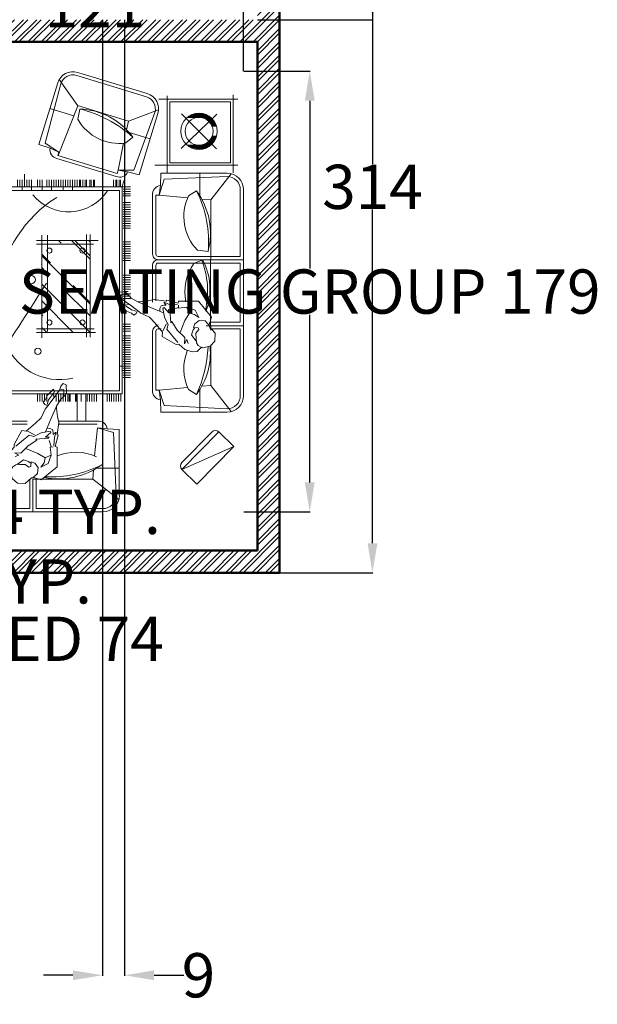
# Model space of a CAD drawing. Units: inches. Extents: x -90 to 536, y -553 to 299.
# Tile 14 of 27: x 301 to 536, y -553 to -153. Entities that reach past the tile are written whole.
import ezdxf

# ---------------------------------------------------------------- set-up
doc = ezdxf.new("R2010")
doc.units = ezdxf.units.IN
for name, color, linetype, lineweight in [('A-ANNO-DIMS', 2, 'Continuous', 18), ('A-WALL-PATT', 252, 'Continuous', 13), ('Furniture', 2, 'Continuous', 18), ('Outer Wall', 1, 'Continuous', 50)]:
    doc.layers.add(name, color=color, linetype=linetype, lineweight=lineweight)
doc.styles.get("Standard").update_dxf_attribs({"font": 'arial.ttf'})
doc.dimstyles.get("Standard").update_dxf_attribs({"dimtxt": 18, "dimasz": 12, "dimexe": 0.18, "dimexo": 0.0625, "dimgap": 0.09, "dimtad": 0, "dimtih": 1, "dimtoh": 1, "dimdec": 0, "dimzin": 0, "dimdsep": 46, "dimlunit": 3, "dimtxsty": 'Standard', "dimcen": 0.09, "dimadec": 0, "dimazin": 0, "dimtfac": 1, "dimtdec": 0, "dimtofl": 0, "dimtmove": 0, "dimatfit": 3, "dimfxl": 1, "dimtolj": 1, "dimtzin": 0, "dimarcsym": 0})

# ---------------------------------------------------------------- blocks, each defined once
blk = doc.blocks.new('A$C4DC51D13')
for p, q in [((3265.3, 2996.2), (1188.4, 2996.2)), ((1895.2, 2134), (1895.2, 2996.2)), ((2559.6, 2996.2), (2559.6, 2617.8)), ((1018.2, 2892.3), (232.2, 2892.3)), ((277.4, 2939.6), (277.4, 2141.8)), ((943, 2103.5), (943, 2936.7)), ((1188.4, 2962.7), (1862.1, 2962.7)), ((1862.1, 2134), (1862.1, 2962.7)), ((1928.3, 2961.6), (2524.2, 2961.6)), ((1928.3, 2134), (1928.3, 2961.6)), ((2524.2, 2961.6), (2524.2, 2658.6)), ((2590.4, 2962.7), (2590.4, 2654.5)), ((3265.3, 2962.7), (2590.4, 2962.7)), ((3778.5, 2897), (3631.2, 2747.3)), ((4008.9, 2375.5), (3778.5, 2897)), ((4156.2, 2525.2), (3778.5, 2897)), ((304, 2865.7), (304, 2253.3)), ((916.4, 2865.7), (304, 2865.7)), ((916.4, 2253.3), (916.4, 2865.7)), ((1022.9, 2163.8), (1022.9, 2830.3)), ((1290.4, 2664.8), (1028, 2870.9)), ((1056, 2830.3), (1081, 2194.8)), ((3163.3, 2664.8), (3425.7, 2870.9)), ((3397.7, 2830.3), (3364.5, 2194.8)), ((3430.8, 2163.8), (3430.8, 2830.3)), ((423.7, 2370.8), (776.6, 2723.7)), ((427.4, 2727.4), (772.8, 2367.1)), ((476.8, 2615), (476.8, 2682.5)), ((481, 2622.2), (481, 2686.2)), ((485.3, 2628.5), (485.3, 2689.7)), ((489.5, 2634.2), (489.5, 2693)), ((493.7, 2639.3), (493.7, 2696.1)), ((497.9, 2644), (497.9, 2699.1)), ((502.2, 2648.3), (502.2, 2701.8)), ((506.4, 2652.2), (506.4, 2704.4)), ((510.6, 2655.8), (510.6, 2706.9)), ((514.9, 2659.2), (514.9, 2709.2)), ((519.1, 2662.3), (519.1, 2711.3)), ((523.3, 2665.1), (523.3, 2713.4)), ((527.5, 2667.8), (527.5, 2715.2)), ((531.8, 2670.2), (531.8, 2717)), ((536, 2672.5), (536, 2718.7)), ((540.2, 2674.6), (540.2, 2720.2)), ((544.4, 2676.5), (544.4, 2721.6)), ((548.7, 2678.2), (548.7, 2722.9)), ((650.1, 2678.8), (650.1, 2723.3)), ((654.3, 2677.1), (654.3, 2722)), ((658.6, 2675.2), (658.6, 2720.7)), ((662.8, 2673.2), (662.8, 2719.2)), ((667, 2671), (667, 2717.6)), ((668.5, 2670.2), (668.5, 2717)), ((671.2, 2668.6), (671.2, 2715.9)), ((672.7, 2667.8), (672.7, 2715.2)), ((675.5, 2666.1), (675.5, 2714)), ((676.9, 2665.1), (676.9, 2713.4)), ((679.7, 2663.3), (679.7, 2712)), ((681.1, 2662.3), (681.1, 2711.3)), ((683.9, 2660.3), (683.9, 2709.9)), ((685.4, 2659.2), (685.4, 2709.2)), ((688.1, 2657), (688.1, 2707.7)), ((689.6, 2655.8), (689.6, 2706.9)), ((692.4, 2653.5), (692.4, 2705.3)), ((693.8, 2652.2), (693.8, 2704.4)), ((696.6, 2649.6), (696.6, 2702.7)), ((698, 2648.3), (698, 2701.8)), ((700.8, 2645.5), (700.8, 2700)), ((702.3, 2644), (702.3, 2699.1)), ((705, 2641), (705, 2697.2)), ((706.5, 2639.3), (706.5, 2696.1)), ((709.3, 2636), (709.3, 2694.1)), ((710.7, 2634.2), (710.7, 2693)), ((713.5, 2630.5), (713.5, 2690.9)), ((714.9, 2628.5), (714.9, 2689.7)), ((717.7, 2624.4), (717.7, 2687.4)), ((719.2, 2622.2), (719.2, 2686.2)), ((722, 2617.6), (722, 2683.8)), ((723.4, 2615), (723.4, 2682.5)), ((4008.9, 2375.5), (3631.2, 2747.3)), ((420.6, 2582.7), (464, 2582.7)), ((421.5, 2587), (465.2, 2587)), ((422.5, 2591.2), (466.5, 2591.2)), ((423.6, 2595.4), (467.9, 2595.4)), ((424.8, 2599.7), (469.6, 2599.7)), ((426.1, 2603.9), (471.3, 2603.9)), ((426.1, 2490.7), (426.1, 2603.9)), ((427.5, 2608.1), (473.3, 2608.1)), ((429.1, 2612.3), (475.4, 2612.3)), ((430.3, 2479), (430.3, 2615.5)), ((430.7, 2616.6), (477.7, 2616.6)), ((432.5, 2620.8), (480.2, 2620.8)), ((434.5, 2469.3), (434.5, 2625.2)), ((434.5, 2625), (482.9, 2625)), ((436.5, 2629.2), (485.8, 2629.2)), ((438.7, 2633.5), (488.9, 2633.5)), ((438.8, 2460.9), (438.8, 2633.6)), ((441, 2637.7), (492.3, 2637.7)), ((443, 2453.4), (443, 2641.1)), ((443.5, 2641.9), (496, 2641.9)), ((446.1, 2646.1), (500, 2646.1)), ((447.2, 2446.7), (447.2, 2647.8)), ((448.9, 2650.4), (504.4, 2650.4)), ((451.5, 2440.6), (451.5, 2654)), ((451.9, 2654.6), (509.2, 2654.6)), ((455.1, 2658.8), (514.4, 2658.8)), ((455.7, 2434.9), (455.7, 2659.6)), ((458.4, 2663.1), (520.2, 2663.1)), ((459.9, 2558.8), (459.9, 2664.9)), ((462, 2667.3), (526.7, 2667.3)), ((464.1, 2583.3), (464.1, 2669.7)), ((465.8, 2671.5), (534.1, 2671.5)), ((468.4, 2596.6), (468.4, 2674.3)), ((469.8, 2675.7), (542.8, 2675.7)), ((472.6, 2606.7), (472.6, 2678.5)), ((489.5, 2667.3), (489.5, 2633.5)), ((657.4, 2675.7), (730.4, 2675.7)), ((734.5, 2671.5), (666.1, 2671.5)), ((666.1, 2671.5), (734.5, 2671.5)), ((738.2, 2667.3), (673.5, 2667.3)), ((673.5, 2667.3), (738.2, 2667.3)), ((741.8, 2663.1), (680, 2663.1)), ((680, 2663.1), (741.8, 2663.1)), ((745.2, 2658.8), (685.8, 2658.8)), ((685.8, 2658.8), (745.2, 2658.8)), ((748.3, 2654.6), (691, 2654.6)), ((691, 2654.6), (748.3, 2654.6)), ((751.3, 2650.4), (695.8, 2650.4)), ((695.8, 2650.4), (751.3, 2650.4)), ((754.1, 2646.1), (700.2, 2646.1)), ((700.2, 2646.1), (754.1, 2646.1)), ((756.7, 2641.9), (704.2, 2641.9)), ((704.2, 2641.9), (756.7, 2641.9)), ((759.2, 2637.7), (707.9, 2637.7)), ((707.9, 2637.7), (759.2, 2637.7)), ((761.5, 2633.5), (711.3, 2633.5)), ((711.3, 2633.5), (761.5, 2633.5)), ((763.7, 2629.2), (714.4, 2629.2)), ((714.4, 2629.2), (763.7, 2629.2)), ((765.8, 2625), (717.3, 2625)), ((767.7, 2620.8), (720, 2620.8)), ((769.5, 2616.6), (722.5, 2616.6)), ((771.1, 2612.3), (724.8, 2612.3)), ((726.2, 2609.7), (726.2, 2679.9)), ((772.7, 2608.1), (726.9, 2608.1)), ((727.6, 2606.7), (727.6, 2678.5)), ((774.1, 2603.9), (728.9, 2603.9)), ((730.4, 2600.3), (730.4, 2675.7)), ((775.4, 2599.7), (730.7, 2599.7)), ((731.9, 2596.6), (731.9, 2674.3)), ((776.6, 2595.4), (732.3, 2595.4)), ((777.7, 2591.2), (733.7, 2591.2)), ((734.6, 2588.4), (734.6, 2671.3)), ((778.7, 2587), (735.1, 2587)), ((736.1, 2583.3), (736.1, 2669.7)), ((779.6, 2582.7), (736.2, 2582.7)), ((738.9, 2570.4), (738.9, 2666.6)), ((740.3, 2558.8), (740.3, 2664.9)), ((743.1, 2433.1), (743.1, 2661.5)), ((744.5, 2434.9), (744.5, 2659.6)), ((747.3, 2438.6), (747.3, 2656)), ((748.8, 2440.6), (748.8, 2654)), ((751.5, 2444.5), (751.5, 2650)), ((753, 2446.7), (753, 2647.8)), ((755.8, 2451.1), (755.8, 2643.5)), ((757.2, 2453.4), (757.2, 2641.1)), ((760, 2458.3), (760, 2636.3)), ((761.4, 2460.9), (761.4, 2633.6)), ((764.2, 2466.3), (764.2, 2628.2)), ((765.7, 2469.3), (765.7, 2625.2)), ((1283.3, 2574.2), (1290.4, 2664.8)), ((1290.4, 2664.8), (1894.7, 2664.8)), ((1798, 2530.2), (1812.1, 2637.9)), ((1895.2, 2663.7), (2557.3, 2663.7)), ((1895.5, 2582.2), (1932.3, 2494.6)), ((2603.6, 2664.8), (2559, 2664.8)), ((3163.3, 2664.8), (2764.7, 2664.8)), ((3170.4, 2574.2), (3163.3, 2664.8)), ((3631.7, 2676.6), (3938.2, 2375)), ((417.1, 2548.9), (459.4, 2548.9)), ((417.1, 2544.7), (459.5, 2544.7)), ((417.2, 2553.2), (459.6, 2553.2)), ((417.2, 2540.5), (459.6, 2540.5)), ((417.4, 2557.4), (459.8, 2557.4)), ((417.5, 2536.3), (459.9, 2536.3)), ((417.7, 2561.6), (460.2, 2561.6)), ((417.8, 2532), (460.3, 2532)), ((418.1, 2565.8), (460.7, 2565.8)), ((418.2, 2527.8), (460.8, 2527.8)), ((418.5, 2570.1), (461.3, 2570.1)), ((418.7, 2523.6), (461.4, 2523.6)), ((419.1, 2574.3), (462.1, 2574.3)), ((419.3, 2519.4), (462.2, 2519.4)), ((419.8, 2578.5), (462.9, 2578.5)), ((459.9, 2429.7), (459.9, 2535.7)), ((780.4, 2578.5), (737.3, 2578.5)), ((781, 2519.4), (738, 2519.4)), ((781.1, 2574.3), (738.2, 2574.3)), ((781.6, 2523.6), (738.8, 2523.6)), ((781.7, 2570.1), (738.9, 2570.1)), ((782.1, 2527.8), (739.4, 2527.8)), ((782.2, 2565.8), (739.6, 2565.8)), ((782.5, 2532), (740, 2532)), ((782.5, 2561.6), (740.1, 2561.6)), ((740.3, 2429.7), (740.3, 2535.7)), ((782.8, 2557.4), (740.4, 2557.4)), ((782.8, 2536.3), (740.4, 2536.3)), ((783, 2540.5), (740.6, 2540.5)), ((783, 2553.2), (740.7, 2553.2)), ((783.1, 2548.9), (740.8, 2548.9)), ((783.1, 2544.7), (740.8, 2544.7)), ((1022.9, 2554.4), (1249.6, 2554.4)), ((1200, 2520.5), (1251.9, 2440.8)), ((2559, 2535.8), (2557.3, 2535.8)), ((3253.7, 2520.5), (3201.8, 2440.8)), ((3430.8, 2554.4), (3204.1, 2554.4)), ((4008.9, 2375.5), (4156.2, 2525.2)), ((1243.2, 2146.7), (1272.2, 2431.8)), ((3210.5, 2146.7), (3181.5, 2431.8)), ((242.9, 2226.7), (1018.2, 2226.7)), ((304, 2253.3), (916.4, 2253.3)), ((1081, 2194.8), (1243.2, 2146.7)), ((3364.5, 2194.8), (3210.5, 2146.7)), ((498.8, 1837.1), (382.1, 2139.5)), ((411.8, 2101.9), (992.6, 1890.2)), ((1040.3, 1942.9), (421.2, 2132.6)), ((1145.1, 2159.3), (1022.9, 2163.8)), ((1145.1, 2159.3), (1243.2, 2146.7)), ((1244.8, 2113), (1243.2, 2146.7)), ((1839.5, 2113), (1244.8, 2113)), ((2308.5, 2111.9), (1950.4, 2111.9)), ((2590.4, 2164.3), (2590.4, 2134)), ((2614.2, 2113), (3208.9, 2113)), ((3208.9, 2113), (3210.5, 2146.7)), ((3308.6, 2159.3), (3210.5, 2146.7)), ((3308.6, 2159.3), (3430.8, 2163.8)), ((220.3, 2026), (19.3, 1370.1)), ((251.1, 2016.6), (37.1, 1314.7)), ((677.4, 2054.1), (612.9, 1843.6)), ((1839.5, 2079.9), (1244.8, 2079.9)), ((2322.1, 2078.8), (1950.4, 2078.8)), ((2614.2, 2079.9), (3208.9, 2079.9)), ((992.6, 1890.2), (993.4, 1733.4)), ((1009.7, 1828.1), (1040.3, 1942.9)), ((498.8, 1837.1), (341.4, 1323.6)), ((584.9, 1817.9), (498.8, 1837.1)), ((658.5, 1880), (717.8, 1809.1)), ((993.4, 1733.4), (720.4, 1787.6)), ((1009.7, 1828.1), (993.4, 1733.4)), ((1166.1, 1769.7), (1091.8, 1794.5)), ((1158.3, 1784.3), (1158.3, 1858.2)), ((1158.3, 1821.3), (1158.5, 487.7)), ((1181.8, 1784.3), (1181.8, 1858.2)), ((1205.3, 1784.3), (1205.3, 1858.2)), ((1228.8, 1784.3), (1228.8, 1858.2)), ((1252.2, 1784.3), (1252.2, 1858.2)), ((1319.4, 1784.3), (1319.4, 1858.2)), ((1342.9, 1784.3), (1342.9, 1858.2)), ((1366.3, 1784.3), (1366.3, 1858.2)), ((1389.8, 1784.3), (1389.8, 1858.2)), ((1413.3, 1784.3), (1413.3, 1858.2)), ((1436.8, 1784.3), (1436.8, 1858.2)), ((1460.2, 1784.3), (1460.2, 1858.2)), ((1483.7, 1784.3), (1483.7, 1858.2)), ((1507.2, 1784.3), (1507.2, 1858.2)), ((1530.7, 1784.3), (1530.7, 1858.2)), ((1554.1, 1784.3), (1554.1, 1858.2)), ((1577.6, 1784.3), (1577.6, 1858.2)), ((1714.2, 1784.3), (1714.2, 1858.2)), ((1737.6, 1784.3), (1737.6, 1858.2)), ((1761.1, 1784.3), (1761.1, 1858.2)), ((1784.6, 1784.3), (1784.6, 1858.2)), ((1808.1, 1784.3), (1808.1, 1858.2)), ((1831.5, 1784.3), (1831.5, 1858.2)), ((1855, 1784.3), (1855, 1858.2)), ((1878.5, 1784.3), (1878.5, 1858.2)), ((1902, 1784.3), (1902, 1858.2)), ((2050.7, 1784.3), (2050.7, 1858.2)), ((2074.2, 1784.3), (2074.2, 1858.2)), ((2097.7, 1784.3), (2097.7, 1858.2)), ((2121.1, 1784.3), (2121.1, 1858.2)), ((2144.6, 1784.3), (2144.6, 1858.2)), ((2168.1, 1784.3), (2168.1, 1858.2)), ((2191.6, 1782.4), (2191.6, 1856.3)), ((2215, 1785.7), (2215, 1832.3)), ((2238.5, 1785.1), (2238.5, 1859)), ((2262, 1784.3), (2262, 1858.2)), ((2285.4, 1784.3), (2285.4, 1858.2)), ((2543.7, 1784.3), (2543.7, 1858.2)), ((2567.1, 1784.3), (2567.1, 1858.2)), ((2590.6, 1784.3), (2590.6, 1858.2)), ((2614.1, 1784.3), (2614.1, 1858.2)), ((2661, 1784.3), (2661, 1858.2)), ((2684.5, 1784.3), (2684.5, 1858.2)), ((2708, 1772.3), (2708, 1858.2)), ((2731.5, 1784.3), (2731.5, 1858.2)), ((2754.9, 1784.3), (2754.9, 1858.2)), ((2778.4, 1784.3), (2778.4, 1858.2)), ((2801.9, 1784.3), (2801.9, 1858.2)), ((2825.4, 1784.3), (2825.4, 1858.2)), ((2848.8, 1784.3), (2848.8, 1858.2)), ((2872.3, 1784.3), (2872.3, 1858.2)), ((2895.8, 1784.3), (2895.8, 1858.2)), ((2919.3, 1784.3), (2919.3, 1858.2)), ((2942.7, 1784.3), (2942.7, 1858.2)), ((2966.2, 1744.8), (2966.2, 1858.2)), ((2989.7, 1784.3), (2989.7, 1858.2)), ((3013.2, 1772.3), (3013.2, 1858.2)), ((3036.6, 1784.3), (3036.6, 1858.2)), ((3060.1, 1784.3), (3060.1, 1858.2)), ((3083.6, 1784.3), (3083.6, 1858.2)), ((1024.2, 1722.3), (842.3, 1125.2)), ((873.1, 1115.8), (1055, 1712.9)), ((1024.2, 1722.3), (993.4, 1733.4)), ((1162.1, 1754.9), (1088.2, 1754.9)), ((1162.1, 1741.1), (1088.2, 1741.1)), ((1162.1, 1717.6), (1088.2, 1717.6)), ((1162.1, 1708), (1088.2, 1708)), ((3248.4, 1772.3), (1158.5, 1772.3)), ((1196, 511), (1196, 1744.8)), ((1196, 1744.8), (3215.6, 1744.8)), ((3215.6, 511), (3215.6, 1744.8)), ((3248.4, 487.7), (3248.4, 1772.3)), ((3248.8, 1760.8), (3322.7, 1760.8)), ((3248.8, 1737.3), (3322.7, 1737.3)), ((3248.8, 1713.8), (3322.7, 1713.8)), ((3248.8, 1690.4), (3322.7, 1690.4)), ((3600.6, 1621.7), (3605.1, 1743.8)), ((3605.1, 1743.8), (4271.6, 1743.8)), ((4271.6, 1710.7), (3636.1, 1685.8)), ((3995.7, 1743.8), (3995.7, 1517.1)), ((4106.1, 1476.4), (4312.2, 1738.8)), ((1162.1, 1684.5), (1088.2, 1684.5)), ((3248.8, 1666.9), (3322.7, 1666.9)), ((3248.8, 1643.4), (3322.7, 1643.4)), ((3248.8, 1619.9), (3322.7, 1619.9)), ((3636.1, 1685.8), (3588, 1523.6)), ((3600.6, 1621.7), (3588, 1523.6)), ((1162.1, 1492.9), (1088.2, 1492.9)), ((1701.7, 1530), (1701.7, 911.2)), ((2593.1, 907.9), (2593.1, 1490.3)), ((2629.1, 907.9), (2629.1, 1503.1)), ((3248.8, 1513.8), (3322.7, 1513.8)), ((3248.8, 1513.3), (3322.7, 1513.3)), ((3248.8, 1490.4), (3322.7, 1490.4)), ((3248.8, 1489.9), (3322.7, 1489.9)), ((3521.2, 1130.7), (3521.2, 1521.9)), ((3554.3, 1131.4), (3554.3, 1521.9)), ((3588, 1523.6), (3873.1, 1494.5)), ((4404, 1578.3), (4404, 904.6)), ((4437.5, 165.9), (4437.5, 1578.3)), ((1162.1, 1483.3), (1088.2, 1483.3)), ((1162.1, 1459.8), (1088.2, 1459.8)), ((1162.1, 1446), (1088.2, 1446)), ((1162.1, 1412.8), (1088.2, 1412.8)), ((1162.1, 1399), (1088.2, 1399)), ((2674.6, 1449.9), (1641, 1449.9)), ((2674.6, 1413.9), (1641, 1413.9)), ((1888.1, 1449.9), (1701.7, 1263.5)), ((1856.2, 1449.9), (1701.7, 1295.4)), ((1715.1, 1449.9), (1701.7, 1436.5)), ((1737.7, 1483.1), (1737.7, 911.2)), ((2343.3, 1449.9), (1855.3, 961.9)), ((2629.1, 1449), (2142, 961.9)), ((2325.1, 1449.9), (2154.2, 1279.1)), ((2461.6, 1449.9), (2177, 1165.3)), ((3248.8, 1466.9), (3322.7, 1466.9)), ((3248.8, 1443.4), (3322.7, 1443.4)), ((3248.8, 1419.9), (3322.7, 1419.9)), ((3250, 1407.8), (3519, 1407.8)), ((4015.5, 1483.4), (4106.1, 1476.4)), ((4106.1, 1476.4), (4106.1, 872.1)), ((6.3, 1324.2), (19.3, 1370.2)), ((342.8, 1324.6), (76.7, 1139.6)), ((843, 1127.6), (342.8, 1324.6)), ((479.3, 1327.3), (375.2, 1344.9)), ((1162.1, 1375.5), (1088.2, 1375.5)), ((1162.1, 1352.1), (1088.2, 1352.1)), ((1162.1, 1342.9), (1088.2, 1342.9)), ((1162.1, 1342.4), (1088.2, 1342.4)), ((1162.1, 1319.4), (1088.2, 1319.4)), ((1162.1, 1318.9), (1088.2, 1318.9)), ((1162.1, 1296), (1088.2, 1296)), ((1162.1, 1295.5), (1088.2, 1295.5)), ((3248.8, 990.8), (3248.4, 1328.4)), ((3248.8, 1359), (3322.7, 1359)), ((3248.8, 1312.1), (3322.7, 1312.1)), ((3248.8, 1302.3), (3322.7, 1302.3)), ((3250, 1317.8), (3519, 1317.8)), ((369.2, 1044.8), (442.9, 1285.2)), ((1196, 1272.5), (1088.2, 1272.5)), ((1162.1, 1272), (1088.2, 1272)), ((1162.1, 1249), (1088.2, 1249)), ((1162.1, 1248.5), (1088.2, 1248.5)), ((1162.1, 1225.5), (1088.2, 1225.5)), ((1162.1, 1202.1), (1088.2, 1202.1)), ((2629.1, 1280.5), (2310.5, 961.9)), ((3248.8, 1249), (3322.7, 1249)), ((3248.8, 1248.5), (3322.7, 1248.5)), ((3248.8, 1239.3), (3322.7, 1239.3)), ((3248.8, 1238.8), (3322.7, 1238.8)), ((3248.8, 1225.5), (3322.7, 1225.5)), ((3248.8, 1202.1), (3322.7, 1202.1)), ((732, 933.5), (112.9, 1123.3)), ((122.4, 1154.1), (719.7, 996.3)), ((719.7, 996.3), (810.6, 1133.2)), ((771, 1045.7), (810.6, 1133.2)), ((842.3, 1125.2), (810.6, 1133.2)), ((1196, 1178.6), (1088.2, 1178.6)), ((1162.1, 1155.1), (1088.2, 1155.1)), ((1162.1, 1131.6), (1088.2, 1131.6)), ((1162.1, 1108.2), (1088.2, 1108.2)), ((1728.6, 1158.4), (1701.7, 1131.5)), ((3248.8, 1178.6), (3322.7, 1178.6)), ((3248.8, 1155.1), (3322.7, 1155.1)), ((3248.8, 1131.6), (3322.7, 1131.6)), ((3248.8, 1108.2), (3322.7, 1108.2)), ((771, 1045.7), (732, 933.5)), ((1162.1, 1084.7), (1088.2, 1084.7)), ((1196, 1061.2), (1088.2, 1061.2)), ((1162.1, 1037.7), (1088.2, 1037.7)), ((1162.1, 1014.3), (1088.2, 1014.3)), ((1648.3, 1019.6), (2616.7, 1019.6)), ((1926.6, 1051.5), (1837.1, 961.9)), ((2006.3, 994.6), (1973.6, 961.9)), ((2629.1, 1012), (2579, 961.9)), ((3248.8, 1014.3), (3322.7, 1014.3)), ((1196, 967.3), (1088.2, 967.3)), ((1162.1, 943.8), (1088.2, 943.8)), ((1162.1, 920.4), (1088.2, 920.4)), ((1648.3, 961.9), (2681.9, 961.9)), ((2459.2, 974.1), (2447, 961.9)), ((3248.8, 990.8), (3322.7, 990.8)), ((3248.8, 967.3), (3322.7, 967.3)), ((3248.8, 943.8), (3322.7, 943.8)), ((3248.8, 920.4), (3322.7, 920.4)), ((4097.4, 904.6), (4404, 904.6)), ((1196, 860.5), (1088.2, 860.5)), ((1162.1, 837), (1088.2, 837)), ((1162.1, 813.5), (1088.2, 813.5)), ((3521.2, 816.9), (3521.2, 222.3)), ((3554.3, 816.9), (3554.3, 222.3)), ((4106.1, 871.5), (4437.5, 871.5)), ((4404, 840.7), (4110.5, 840.7)), ((4404, 165.9), (4404, 840.7)), ((1162.1, 790), (1031.8, 790)), ((1196, 766.6), (1088.2, 766.6)), ((1162.1, 743.1), (1088.2, 743.1)), ((1162.1, 719.6), (1088.2, 719.6)), ((1162.1, 627.8), (1088.2, 627.8)), ((1162.1, 604.4), (1088.2, 604.4)), ((3248.8, 627.8), (3322.7, 627.8)), ((3248.8, 604.4), (3322.7, 604.4)), ((4106.1, 267.8), (4106.1, 666.5)), ((1162.1, 580.9), (1034.2, 580.9)), ((1162.1, 557.4), (1088.2, 557.4)), ((1162.1, 533.9), (1088.2, 533.9)), ((1162.1, 510.5), (1088.2, 510.5)), ((3215.6, 511), (1196, 511)), ((1334.6, 511), (1334.6, 402.4)), ((1381.6, 511), (1381.6, 402.4)), ((2059.5, 511), (2059.5, 402.4)), ((2106.4, 511), (2106.4, 402.4)), ((2669.8, 511), (2669.8, 402.4)), ((3248.8, 580.9), (3322.7, 580.9)), ((3248.8, 557.4), (3322.7, 557.4)), ((3248.8, 533.9), (3322.7, 533.9)), ((3248.8, 510.5), (3322.7, 510.5)), ((1162, 495.1), (1116.6, 429)), ((1158.5, 487.7), (3248.4, 487.7)), ((1167.1, 476.3), (1167.1, 402.4)), ((1190.6, 476.3), (1190.6, 402.4)), ((1214, 476.3), (1214, 402.4)), ((1237.5, 476.3), (1237.5, 402.4)), ((1311.1, 487.7), (1311.1, 402.4)), ((1358.1, 476.3), (1358.1, 402.4)), ((1405, 476.3), (1405, 402.4)), ((1428.5, 487.7), (1428.5, 402.4)), ((1452, 476.3), (1452, 402.4)), ((1475.5, 476.3), (1475.5, 402.4)), ((1498.9, 487.7), (1498.9, 402.4)), ((1522.4, 487.7), (1522.4, 402.4)), ((1545.9, 476.3), (1545.9, 402.4)), ((1569.4, 476.3), (1569.4, 402.4)), ((1592.8, 476.3), (1592.8, 402.4)), ((1616.3, 476.3), (1616.3, 402.4)), ((1639.8, 476.3), (1639.8, 402.4)), ((1663.3, 487.7), (1663.3, 402.4)), ((1757.8, 487.7), (1757.8, 402.4)), ((1781.3, 487.7), (1781.3, 402.4)), ((1804.8, 476.3), (1804.8, 402.4)), ((1828.2, 476.3), (1828.2, 402.4)), ((1851.7, 476.3), (1851.7, 402.4)), ((1875.2, 476.3), (1875.2, 402.4)), ((1898.7, 476.3), (1898.7, 402.4)), ((1922.1, 487.7), (1922.1, 402.4)), ((2036, 487.7), (2036, 402.4)), ((2082.9, 476.3), (2082.9, 402.4)), ((2129.9, 476.3), (2129.9, 402.4)), ((2153.4, 487.7), (2153.4, 402.4)), ((2176.8, 476.3), (2176.8, 402.4)), ((2200.3, 476.3), (2200.3, 402.4)), ((2223.8, 487.7), (2223.8, 402.4)), ((2247.2, 487.7), (2247.2, 402.4)), ((2270.7, 476.3), (2270.7, 402.4)), ((2294.2, 476.3), (2294.2, 402.4)), ((2317.7, 476.3), (2317.7, 402.4)), ((2341.1, 476.3), (2341.1, 402.4)), ((2364.6, 476.3), (2364.6, 402.4)), ((2388.1, 487.7), (2388.1, 402.4)), ((2411.6, 476.3), (2411.6, 402.4)), ((2435, 476.3), (2435, 402.4)), ((2458.5, 476.3), (2458.5, 402.4)), ((2482, 487.7), (2482, 402.4)), ((2505.5, 487.7), (2505.5, 402.4)), ((2528.9, 476.3), (2528.9, 402.4)), ((2552.4, 476.3), (2552.4, 402.4)), ((2575.9, 476.3), (2575.9, 402.4)), ((2599.4, 476.3), (2599.4, 402.4)), ((2622.8, 476.3), (2622.8, 402.4)), ((2646.3, 476.3), (2646.3, 402.4)), ((2693.3, 476.3), (2693.3, 402.4)), ((2716.7, 476.3), (2716.7, 402.4)), ((2738, 476.3), (2738, 402.4)), ((2740.2, 487.7), (2740.2, 402.4)), ((2761.5, 476.3), (2761.5, 402.4)), ((2763.7, 476.3), (2763.7, 402.4)), ((2784.9, 487.7), (2784.9, 402.4)), ((2787.2, 476.3), (2787.2, 402.4)), ((2808.4, 476.3), (2808.4, 402.4)), ((2810.6, 476.3), (2810.6, 402.4)), ((2831.9, 476.3), (2831.9, 402.4)), ((2834.1, 476.3), (2834.1, 402.4)), ((2855.4, 476.3), (2855.4, 402.4)), ((2857.6, 476.3), (2857.6, 402.4)), ((2878.8, 476.3), (2878.8, 402.4)), ((2881.1, 476.3), (2881.1, 402.4)), ((2902.3, 476.3), (2902.3, 402.4)), ((2904.5, 487.7), (2904.5, 402.4)), ((2925.8, 476.3), (2925.8, 402.4)), ((2928, 476.3), (2928, 402.4)), ((2949.3, 476.3), (2949.3, 402.4)), ((2951.5, 476.3), (2951.5, 402.4)), ((2972.7, 476.3), (2972.7, 402.4)), ((2975, 476.3), (2975, 402.4)), ((2996.2, 476.3), (2996.2, 402.4)), ((2998.4, 476.3), (2998.4, 402.4)), ((3019.7, 476.3), (3019.7, 402.4)), ((3021.9, 487.7), (3021.9, 402.4)), ((3043.2, 476.3), (3043.2, 402.4)), ((3045.4, 476.3), (3045.4, 402.4)), ((3066.6, 476.3), (3066.6, 402.4)), ((3068.9, 476.3), (3068.9, 402.4)), ((3092.3, 476.3), (3092.3, 402.4)), ((3092.7, 484.5), (3092.7, 410.6)), ((3115.8, 476.3), (3115.8, 402.4)), ((3116.2, 484.5), (3116.2, 410.6)), ((3202.2, 476.3), (3202.2, 402.4)), ((3225.7, 476.3), (3225.7, 402.4)), ((3244.9, 495.1), (3290.3, 429)), ((3249.2, 476.3), (3249.2, 402.4)), ((3588, 220.6), (3873.1, 249.7)), ((3636.1, 66.6), (3588, 220.6)), ((3961.8, 177.4), (3882.1, 229.3)), ((3995.7, 0.4), (3995.7, 227)), ((4015.5, 260.8), (4106.1, 267.8)), ((4106.1, 267.8), (4312.2, 5.4)), ((3600.6, 122.5), (3605.1, 0.4)), ((3605.1, 0.4), (4271.6, 0.4)), ((4271.6, 33.5), (3636.1, 66.6))]:
    blk.add_line(p, q)
at = {"linetype": 'ByBlock'}
for points in [[(2342.9, 1843.9), (2352.5, 1810.4), (2340.1, 1777.7), (2351.8, 1757), (2412.3, 1818), (2433.1, 1866.4), (2453.1, 1889.5), (2436, 1914.7), (2407.6, 1926.2), (2433.7, 1959.9), (2473.1, 2048.3), (2530.6, 2101.1), (2625.9, 2180.3), (2669, 2174.2), (2748.1, 2315.4), (2745.8, 2342.6), (2801.2, 2404.9), (2823.9, 2479.6), (2818.4, 2529.9), (2775.1, 2571.7), (2782.4, 2583.3), (2765.2, 2658.8), (2714.5, 2706.9), (2634.6, 2708.6), (2571.9, 2652.6), (2548.8, 2649.4), (2474, 2672.1), (2312.9, 2542.1), (2312.9, 2341.6), (2333.9, 2336.4), (2302, 2223.9), (2313.6, 2216.6), (2297.4, 2095.7), (2309.3, 2034.9), (2320.2, 1952), (2319.3, 1929.9), (2280.8, 1863.6), (2257.7, 1842.4), (2239.2, 1825.7), (2220.1, 1798.2), (2221.6, 1713.1), (2254.3, 1700.7), (2275.9, 1729.8), (2288.6, 1768), (2313.7, 1797.6)], [(3285.2, 1088.3), (3251.7, 1078.6), (3219, 1091.1), (3198.3, 1079.4), (3259.3, 1018.8), (3307.7, 998), (3330.8, 978), (3356, 995.1), (3367.5, 1023.6), (3401.2, 997.5), (3489.6, 958), (3542.4, 900.5), (3621.6, 805.3), (3615.5, 762.2), (3756.7, 683), (3783.9, 685.3), (3846.2, 629.9), (3920.9, 607.2), (3971.2, 612.7), (4013, 656), (4024.6, 648.7), (4100.1, 665.9), (4148.2, 716.6), (4149.9, 796.5), (4093.9, 859.3), (4090.7, 882.4), (4113.4, 957.1), (3983.4, 1118.2), (3782.9, 1118.2), (3777.7, 1097.2), (3665.2, 1129.2), (3657.9, 1117.6), (3537, 1133.7), (3476.2, 1121.9), (3393.3, 1110.9), (3371.2, 1111.9), (3304.9, 1150.4), (3283.7, 1173.4), (3267, 1191.9), (3239.5, 1211), (3154.4, 1209.5), (3142, 1176.8), (3171.1, 1155.3), (3209.3, 1142.5), (3238.9, 1117.5)]]:
    blk.add_lwpolyline(points, close=True, dxfattribs=at)
for points in [[(2563.4, 2654.7), (2512.2, 2609.3), (2506.2, 2548.3), (2540.1, 2504.4), (2576.9, 2490.9), (2579.8, 2539.3), (2598.7, 2543.6), (2636.7, 2516.4), (2690.3, 2516.7), (2731.2, 2520.1), (2758.5, 2540.1), (2773, 2563.3)], [(2629.1, 2357.8), (2507, 2405.5), (2433.2, 2450.3), (2445.5, 2500.8), (2478.9, 2546.1), (2402.4, 2506.9), (2373.4, 2424.8), (2384.4, 2341.9), (2352.8, 2340.7)], [(2712.3, 2515.8), (2652.7, 2472.4), (2603.2, 2489), (2580, 2503.6)], [(2738, 2438.2), (2699.2, 2425.4), (2742.4, 2401.4), (2680.4, 2403.2), (2604.1, 2328.3), (2519.2, 2273.3), (2529.8, 2261.8), (2402.7, 2252.7), (2395.4, 2241.1), (2431.1, 2241.3), (2375.7, 2196.9), (2385.2, 2181.2), (2474.4, 2199.5), (2549.9, 2234.6), (2596.2, 2223.2), (2730.1, 2333.1)], [(2433.2, 2450.3), (2377.6, 2423.8)], [(2409.5, 2153), (2387.5, 2153.9), (2359, 2165.4), (2352.6, 2193.7), (2353.5, 2215.7), (2330.5, 2194.6), (2322.1, 2196.7), (2341.8, 2240.9), (2345.5, 2329.1)], [(2374.9, 2339.8), (2395.2, 2276.9)], [(2431.4, 2187.8), (2379.5, 2066.7), (2320.2, 1929.7)], [(2613.2, 2183.4), (2541.6, 2218.8)], [(2407.6, 1926.2), (2342.9, 1843.9)], [(2412.9, 1911.5), (2401.6, 1865.2), (2361.9, 1812.5)], [(2279.2, 1765.9), (2259.2, 1757.4), (2247.6, 1764.7), (2246.4, 1796.2), (2253.5, 1843.5)], [(3207.2, 1152), (3198.7, 1171.9), (3206, 1183.5), (3237.5, 1184.7), (3284.8, 1177.6)], [(3629.1, 999.7), (3508, 1051.6), (3371, 1110.9)], [(3594.3, 1021.6), (3595.2, 1043.7), (3606.7, 1072.1), (3635, 1078.6), (3657, 1077.6), (3635.9, 1100.6), (3638, 1109.1), (3682.2, 1089.3), (3770.4, 1085.6)], [(3352.8, 1018.2), (3306.5, 1029.5), (3253.8, 1069.2)], [(3367.5, 1023.6), (3285.2, 1088.3)], [(3879.5, 693.2), (3866.7, 732), (3842.7, 688.8), (3844.5, 750.8), (3769.6, 827.1), (3714.6, 911.9), (3703.1, 901.3), (3694, 1028.4), (3682.4, 1035.7), (3682.6, 1000), (3638.2, 1055.5), (3622.5, 1045.9), (3640.8, 956.7), (3675.9, 881.2), (3664.5, 834.9), (3774.4, 701)], [(3781.1, 1056.2), (3718.2, 1035.9)], [(3799.1, 802), (3846.8, 924.2), (3891.6, 998), (3942.1, 985.6), (3987.4, 952.2), (3948.2, 1028.7), (3866.1, 1057.7), (3783.2, 1046.8), (3782, 1078.3)], [(3891.6, 998), (3865.1, 1053.5)], [(4096, 867.7), (4050.6, 918.9), (3989.6, 924.9), (3945.7, 891.1), (3932.2, 854.2), (3980.6, 851.3), (3984.9, 832.4), (3957.7, 794.4), (3958, 740.9), (3961.4, 699.9), (3981.4, 672.7), (4004.6, 658.1)], [(3624.7, 817.9), (3660.1, 889.6)], [(3957.1, 718.8), (3913.7, 778.5), (3930.3, 827.9), (3944.9, 851.1)]]:
    blk.add_lwpolyline(points, dxfattribs=at)
for centre, radius in [((600.1, 2547.3), 183), ((600.1, 2547.3), 140.7), ((1803.2, 1372.6), 25.7), ((2527.6, 1372.6), 25.7), ((1803.2, 1039.3), 25.7), ((2527.6, 1039.3), 25.7), ((2095.7, 858), 41), ((2817.9, 923.4), 31.7)]:
    blk.add_circle(centre, radius)
for centre, radius, start, end in [((1188.4, 2830.3), 165.9, 90, 180), ((3265.3, 2830.3), 165.9, 0, 90), ((1188.4, 2830.3), 132.4, 90, 180), ((3265.3, 2830.3), 132.4, 0, 90), ((3666.8, 2712.2), 50, 135.45034, 225.45034), ((1626.8, 1949.8), 712.7, 74.92803, 126.79295), ((1707.9, 1527), 1115.8, 84.64056, 117.08042), ((2210.2, 1780.8), 852.5, 76.86605, 111.68388), ((2192.2, 2032.6), 624.6, 69.41448, 118.36207), ((2633.9, 373.6), 2292.5, 91.87258, 91.91436), ((2832.8, 1963.1), 698.5, 52.93893, 95.07887), ((2713.3, 1357.7), 1282.3, 65.07253, 87.21518), ((1459.9, 2882.7), 488.4, 244.78659, 313.80576), ((2216, 2892.1), 488.4, 234.48878, 282.12853), ((2993.8, 2882.7), 488.4, 248.21522, 295.21341), ((3973.2, 2410.6), 50, 225.45034, 315.45034), ((374.1, 1978.9), 160.8, 72.95712, 162.95712), ((374.1, 1978.9), 128.6, 72.95712, 162.95712), ((1234.5, 2169.3), 90, 186.42508, 276.58214), ((1839.5, 2135.1), 22.1, 270, 0), ((1839.5, 2135.1), 55.2, 270, 0), ((1950.4, 2134), 55.2, 180, 270), ((1950.4, 2134), 22.1, 180, 270), ((2619.6, 2148.3), 68.5, 191.05953, 265.44258), ((2614.2, 2135.1), 22.1, 180, 270), ((3219.2, 2169.3), 90, 263.41786, 353.57492), ((1584.7, 1047), 1245.7, 138.02964, 166.16361), ((1067.1, 1321), 692.3, 126.16417, 178.02908), ((248.2, 1741.7), 474.4, 299.15135, 8.17052), ((974.8, 1747.9), 87.4, 336.37497, 66.53204), ((4271.6, 1578.3), 165.9, 0, 90), ((4271.6, 1578.3), 132.4, 0, 90), ((944.2, 1233.8), 467.1, 309.48045, 56.62096), ((3610.6, 1532.2), 90, 96.42508, 186.58214), ((4324, 1306.8), 488.4, 154.78659, 202.71372), ((3383, 1136.2), 721.4, 348.10461, 36.64421), ((2968.3, 1058.8), 1115.8, 356.75427, 27.08042), ((160.1, 1277), 160.8, 162.95712, 252.95712), ((160.1, 1277), 128.6, 162.95712, 252.95712), ((2517.5, 1143.6), 586.7, 287.33946, 13.14632), ((787.1, 1131.7), 87.4, 259.3822, 349.53926), ((2356.9, 1798.1), 1287.8, 212.11527, 261.93233), ((-29968.2, -49615.7), 59944, 56.743614, 57.623407), ((4324, 437.4), 488.4, 158.21522, 205.21341), ((3404.4, 598.4), 698.5, 322.93893, 5.07887), ((2799, 717.9), 1282.3, 335.07253, 357.21518), ((2591.9, -2109.1), 2694.5, 80.98418, 100.02608), ((3610.6, 212), 90, 173.41786, 263.57492), ((4271.6, 165.9), 132.4, 270, 0), ((4271.6, 165.9), 165.9, 270, 0)]:
    blk.add_arc(centre, radius, start, end)
blk = doc.blocks.new('*D35')
at = {"layer": 'A-ANNO-DIMS', "color": 0, "lineweight": -2, "transparency": 16777216}
for p, q in [((233.19, -331.05), (239.84, -331.05)), ((239.66, -343.05), (239.66, -343.4)), ((239.66, -362.55), (239.66, -362.21)), ((233.19, -374.55), (239.84, -374.55))]:
    blk.add_line(p, q, dxfattribs=at)
at = {"layer": 'A-ANNO-DIMS', "color": 0, "transparency": 16777216}
for points in [[(237.66, -343.05), (241.66, -343.05), (239.66, -331.05)], [(237.66, -362.55), (241.66, -362.55), (239.66, -374.55)]]:
    blk.add_solid(points, dxfattribs=at)
at = {"layer": 'Defpoints', "color": 0, "transparency": 16777216}
for p in [(233.13, -331.05), (239.66, -331.05), (233.13, -374.55)]:
    blk.add_point(p, dxfattribs=at)
at = {"layer": 'A-ANNO-DIMS', "color": 0, "transparency": 16777216, "insert": (239.66, -352.8), "char_height": 18, "attachment_point": 5}
blk.add_mtext('\\A1;ENTRY DOOR 44 TYP.', dxfattribs=at)
blk = doc.blocks.new('*D36')
at = {"layer": 'A-ANNO-DIMS', "color": 0, "lineweight": -2, "transparency": 16777216}
for p, q in [((191.13, -374.62), (191.13, -381.26)), ((233.13, -374.62), (233.13, -381.26)), ((203.13, -381.08), (221.13, -381.08)), ((233.13, -381.08), (245.13, -381.08))]:
    blk.add_line(p, q, dxfattribs=at)
at = {"layer": 'A-ANNO-DIMS', "color": 0, "transparency": 16777216}
for points in [[(203.13, -379.08), (203.13, -383.08), (191.13, -381.08)], [(221.13, -379.08), (221.13, -383.08), (233.13, -381.08)]]:
    blk.add_solid(points, dxfattribs=at)
at = {"layer": 'Defpoints', "color": 0, "transparency": 16777216}
for p in [(191.13, -374.55), (233.13, -374.55), (233.13, -381.08)]:
    blk.add_point(p, dxfattribs=at)
at = {"layer": 'A-ANNO-DIMS', "color": 0, "transparency": 16777216, "insert": (289.39, -381.08), "char_height": 18, "attachment_point": 5}
blk.add_mtext('\\A1;42 TYP.', dxfattribs=at)
blk = doc.blocks.new('*D43')
at = {"layer": 'A-ANNO-DIMS', "color": 0, "lineweight": -2, "transparency": 16777216}
for p, q in [((392.56, -173.5), (419.57, -173.5)), ((419.39, -185.5), (419.39, -253.75)), ((419.39, -340.81), (419.39, -272.56)), ((392.56, -352.81), (419.57, -352.81))]:
    blk.add_line(p, q, dxfattribs=at)
at = {"layer": 'A-ANNO-DIMS', "color": 0, "transparency": 16777216}
for points in [[(417.39, -185.5), (421.39, -185.5), (419.39, -173.5)], [(417.39, -340.81), (421.39, -340.81), (419.39, -352.81)]]:
    blk.add_solid(points, dxfattribs=at)
at = {"layer": 'Defpoints', "color": 0, "transparency": 16777216}
for p in [(392.5, -173.5), (392.5, -352.81), (419.39, -352.81)]:
    blk.add_point(p, dxfattribs=at)
at = {"layer": 'A-ANNO-DIMS', "color": 0, "transparency": 16777216, "insert": (419.39, -263.15), "char_height": 18, "attachment_point": 5}
blk.add_mtext('\\A1;SEATING GROUP 179', dxfattribs=at)
blk = doc.blocks.new('*D44')
at = {"layer": 'A-ANNO-DIMS', "color": 0, "lineweight": -2, "transparency": 16777216}
for p, q in [((271.59, -173.44), (271.59, -146.42)), ((283.59, -146.6), (314.65, -146.6)), ((380.5, -146.6), (349.43, -146.6)), ((392.5, -173.44), (392.5, -146.42))]:
    blk.add_line(p, q, dxfattribs=at)
at = {"layer": 'A-ANNO-DIMS', "color": 0, "transparency": 16777216}
for points in [[(283.59, -144.6), (283.59, -148.6), (271.59, -146.6)], [(380.5, -144.6), (380.5, -148.6), (392.5, -146.6)]]:
    blk.add_solid(points, dxfattribs=at)
at = {"layer": 'Defpoints', "color": 0, "transparency": 16777216}
for p in [(392.5, -146.6), (271.59, -173.5), (392.5, -173.5)]:
    blk.add_point(p, dxfattribs=at)
at = {"layer": 'A-ANNO-DIMS', "color": 0, "transparency": 16777216, "insert": (332.04, -146.6), "char_height": 18, "attachment_point": 5}
blk.add_mtext('\\A1;121', dxfattribs=at)
blk = doc.blocks.new('*D51')
at = {"layer": 'A-ANNO-DIMS', "color": 0, "lineweight": -2, "transparency": 16777216}
for p, q in [((96.81, -393.34), (96.81, -404.61)), ((171.13, -393.34), (171.13, -404.61)), ((108.81, -404.43), (159.13, -404.43)), ((171.13, -404.43), (183.13, -404.43))]:
    blk.add_line(p, q, dxfattribs=at)
at = {"layer": 'A-ANNO-DIMS', "color": 0, "transparency": 16777216}
for points in [[(108.81, -402.43), (108.81, -406.43), (96.81, -404.43)], [(159.13, -402.43), (159.13, -406.43), (171.13, -404.43)]]:
    blk.add_solid(points, dxfattribs=at)
at = {"layer": 'Defpoints', "color": 0, "transparency": 16777216}
for p in [(96.81, -393.28), (171.13, -393.28), (171.13, -404.43)]:
    blk.add_point(p, dxfattribs=at)
at = {"layer": 'A-ANNO-DIMS', "color": 0, "transparency": 16777216, "insert": (274.99, -404.43), "char_height": 18, "attachment_point": 5}
blk.add_mtext('\\A1;SINGLE BED 74', dxfattribs=at)
blk = doc.blocks.new('*D55')
at = {"layer": 'A-ANNO-DIMS', "color": 0, "lineweight": -2, "transparency": 16777216}
for p, q in [((398.19, -71.55), (445.07, -71.55)), ((444.89, -83.55), (444.89, -102.77)), ((444.89, -140.55), (444.89, -121.33)), ((398.19, -152.55), (445.07, -152.55))]:
    blk.add_line(p, q, dxfattribs=at)
at = {"layer": 'A-ANNO-DIMS', "color": 0, "transparency": 16777216}
for points in [[(442.89, -83.55), (446.89, -83.55), (444.89, -71.55)], [(442.89, -140.55), (446.89, -140.55), (444.89, -152.55)]]:
    blk.add_solid(points, dxfattribs=at)
at = {"layer": 'Defpoints', "color": 0, "transparency": 16777216}
for p in [(398.13, -71.55), (398.13, -152.55), (444.89, -152.55)]:
    blk.add_point(p, dxfattribs=at)
at = {"layer": 'A-ANNO-DIMS', "color": 0, "transparency": 16777216, "insert": (444.89, -112.05), "char_height": 18, "attachment_point": 5}
blk.add_mtext('\\A1;81', dxfattribs=at)
blk = doc.blocks.new('*D61')
at = {"layer": 'A-ANNO-DIMS', "color": 0, "lineweight": -2, "transparency": 16777216}
for p, q in [((335.13, -152.62), (335.13, -541.49)), ((344.13, -152.62), (344.13, -541.49)), ((323.13, -541.31), (311.13, -541.31)), ((356.13, -541.31), (368.13, -541.31))]:
    blk.add_line(p, q, dxfattribs=at)
at = {"layer": 'A-ANNO-DIMS', "color": 0, "transparency": 16777216}
for points in [[(323.13, -539.31), (323.13, -543.31), (335.13, -541.31)], [(356.13, -539.31), (356.13, -543.31), (344.13, -541.31)]]:
    blk.add_solid(points, dxfattribs=at)
at = {"layer": 'Defpoints', "color": 0, "transparency": 16777216}
for p in [(335.13, -152.55), (344.13, -152.55), (344.13, -541.31)]:
    blk.add_point(p, dxfattribs=at)
at = {"layer": 'A-ANNO-DIMS', "color": 0, "transparency": 16777216, "insert": (374.14, -541.31), "char_height": 18, "attachment_point": 5}
blk.add_mtext('\\A1;9', dxfattribs=at)
blk = doc.blocks.new('*D68')
at = {"layer": 'A-ANNO-DIMS', "color": 0, "lineweight": -2, "transparency": 16777216}
for p, q in [((407.19, -63.55), (445.07, -63.55)), ((444.89, -75.55), (444.89, -211.27)), ((444.89, -365.55), (444.89, -229.84)), ((407.19, -377.55), (445.07, -377.55))]:
    blk.add_line(p, q, dxfattribs=at)
at = {"layer": 'A-ANNO-DIMS', "color": 0, "transparency": 16777216}
for points in [[(442.89, -75.55), (446.89, -75.55), (444.89, -63.55)], [(442.89, -365.55), (446.89, -365.55), (444.89, -377.55)]]:
    blk.add_solid(points, dxfattribs=at)
at = {"layer": 'Defpoints', "color": 0, "transparency": 16777216}
for p in [(407.13, -63.55), (407.13, -377.55), (444.89, -377.55)]:
    blk.add_point(p, dxfattribs=at)
at = {"layer": 'A-ANNO-DIMS', "color": 0, "transparency": 16777216, "insert": (444.89, -220.55), "char_height": 18, "attachment_point": 5}
blk.add_mtext('\\A1;314', dxfattribs=at)

msp = doc.modelspace()

# ---------------------------------------------------------------- hatches: boundary and pattern name
at = {"layer": 'A-WALL-PATT'}
h = msp.add_hatch(dxfattribs=at)
h.set_pattern_fill('ANSI32', color=256, scale=0.4)
h.set_pattern_definition([(45, (-88.8105, -603.6155), (-2.694077, 2.694077), []), (45, (-87.0145, -603.6155), (-2.694077, 2.694077), [])])
h.paths.add_polyline_path([(285.1317, 246.4462), (131.1317, 246.4462), (131.1317, 237.4462), (285.1317, 237.4462)])
h.paths.add_polyline_path([(122.1317, 237.4462), (113.1317, 237.4462), (113.1317, 152.4462), (122.1317, 152.4462), (122.1317, 166.4704)])
h.paths.add_polyline_path([(303.1317, 237.4462), (294.1317, 237.4462), (294.1317, 152.4462), (303.1317, 152.4462)])
h.paths.add_polyline_path([(47.1317, 91.9277), (38.1317, 91.9277), (38.1317, -6.5538), (77.1317, -6.5538), (77.1317, 2.4462), (70.5655, 2.4462), (47.1317, 2.4462)])
h.paths.add_polyline_path([(83.052, -61.5538), (47.1317, -61.5538), (47.1317, -24.5538), (38.1317, -24.5538), (38.1317, -70.5538), (74.052, -70.5538), (74.052, -223.5538), (38.1317, -223.5538), (38.1317, -503.5538), (92.1317, -503.5538), (92.1317, -437.5538), (191.1317, -437.5538), (191.1317, -428.5538), (83.1317, -428.5538), (83.1317, -494.5538), (47.1317, -494.5538), (47.1317, -232.5538), (83.052, -232.5538), (83.052, -70.5538)])
h.paths.add_polyline_path([(407.1317, -63.5538), (381.1317, -63.5538), (381.1317, 91.9277), (372.1317, 91.9277), (372.1317, 32.8805), (372.1317, -63.5538), (306.5745, -63.5538), (237.1317, -63.5538), (237.1317, -38.5538), (233.1317, -38.5538), (233.1317, -71.5538), (398.1317, -71.5538), (398.1317, -152.5538), (233.1317, -152.5538), (233.1317, -161.5538), (398.1317, -161.5538), (398.1317, -368.5538), (233.1317, -368.5538), (233.1317, -377.5538), (407.1317, -377.5538), (407.1317, -161.5538)])
h.paths.add_polyline_path([(261.1317, -422.5538), (252.1317, -422.5538), (252.1317, -428.5538), (233.1317, -428.5538), (233.1317, -437.5538), (261.1317, -437.5538)])
h.paths.add_polyline_path([(191.1317, -368.5538), (180.1317, -368.5538), (180.1317, -335.5538), (131.5919, -335.5538), (131.5919, -344.5538), (171.1317, -344.5538), (171.1317, -392.5538), (180.1317, -392.5538), (180.1317, -377.5538), (191.1317, -377.5538)], flags=17)
h.paths.add_polyline_path([(180.1317, -223.5538), (152.1317, -223.5538), (152.1317, -227.5538), (176.1317, -227.5538), (176.1317, -335.5538), (180.1317, -335.5538)], flags=17)
h.paths.add_polyline_path([(131.5919, -335.5538), (83.1317, -335.5538), (83.1317, -339.5538), (83.1317, -392.5538), (87.1317, -392.5538), (87.1317, -339.5538), (131.5919, -339.5538)], flags=17)
h.paths.add_polyline_path([(197.1317, 2.4462), (77.1317, 2.4462), (77.1317, -1.5538), (113.1317, -1.5538), (113.1317, -71.5538), (181.1317, -71.5538), (181.1317, -67.5538), (117.1317, -67.5538), (117.1317, -1.5538), (177.1317, -1.5538), (177.1317, -37.5538), (181.1317, -37.5538), (181.1317, -1.5538), (197.1317, -1.5538)])
h.paths.add_polyline_path([(173.1317, 138.4462), (122.1317, 138.4462), (122.1317, 134.4462), (173.1317, 134.4462)])
h.paths.add_polyline_path([(213.1317, 237.4462), (209.1317, 237.4462), (209.1317, 134.4462), (233.1317, 134.4462), (233.1317, 68.8889), (233.1317, -2.5538), (237.1317, -2.5538), (237.1317, 134.4462), (258.1317, 134.4462), (258.1317, 138.4462), (213.1317, 138.4462)])

# ---------------------------------------------------------------- linework, layer by layer
at = {"layer": 'Outer Wall'}
for p, q in [((407.1317, -161.5538), (407.1317, -63.5538)), ((398.1317, -161.5538), (233.1317, -161.5538)), ((398.1317, -368.5538), (398.1317, -161.5538)), ((407.1317, -377.5538), (407.1317, -161.5538)), ((398.1317, -368.5538), (233.1317, -368.5538)), ((407.1317, -377.5538), (233.1317, -377.5538))]:
    msp.add_line(p, q, dxfattribs=at)

# ---------------------------------------------------------------- block references
at = {"layer": 'Furniture', "xscale": 0.0403522857994069, "yscale": 0.0403522857994069, "zscale": 0.0403522857994069, "rotation": 270}
msp.add_blockref('A$C4DC51D13', (271.5922, -173.7477), dxfattribs=at)

# ---------------------------------------------------------------- dimensions: what is measured, and where the dimension line sits
at = {"layer": 'A-ANNO-DIMS'}
for base, p1, p2, picture, middle in [((444.8867, -377.5538), (407.1317, -63.5538), (407.1317, -377.5538), '*D68', (444.8867, -220.5538)), ((444.8867, -152.5538), (398.1317, -71.5538), (398.1317, -152.5538), '*D55', (444.8867, -112.0538))]:
    dim = msp.add_linear_dim(base=base, p1=p1, p2=p2, angle=90, dimstyle='Standard', override={"dimdec": 0, "dimlfac": 1, "dimrnd": 0, "dimzin": 0, "dimdsep": 46, "dimlunit": 2}, dxfattribs=at)
    dim.commit()
    dim.dimension.update_dxf_attribs({"geometry": picture, "text_midpoint": middle})
for base, p1, p2, picture, middle in [((392.4952, -146.6021), (271.5922, -173.4988), (392.4952, -173.4988), '*D44', (332.0437, -146.6021)), ((344.1317, -541.3088), (335.1317, -152.5538), (344.1317, -152.5538), '*D61', (374.1399, -541.3088))]:
    dim = msp.add_linear_dim(base=base, p1=p1, p2=p2, dimstyle='Standard', override={"dimdec": 0, "dimlfac": 1, "dimrnd": 0, "dimzin": 0, "dimdsep": 46, "dimlunit": 2}, dxfattribs=at)
    dim.commit()
    dim.dimension.update_dxf_attribs({"geometry": picture, "text_midpoint": middle})
for base, p1, p2, angle, text, picture, middle in [((419.392, -352.8104), (392.4952, -173.4988), (392.4952, -352.8104), 270, 'SEATING GROUP <>', '*D43', (419.392, -263.1546)), ((239.6567404714, -331.0537825705), (233.1317404714, -374.5537825705), (233.1317404714, -331.0537825705), 90, 'ENTRY DOOR <> TYP.', '*D35', (239.6567404714, -352.8037825705))]:
    dim = msp.add_linear_dim(base=base, p1=p1, p2=p2, angle=angle, text=text, dimstyle='Standard', override={"dimdec": 0, "dimlfac": 1, "dimrnd": 0, "dimzin": 0, "dimdsep": 46, "dimlunit": 2}, dxfattribs=at)
    dim.commit()
    dim.dimension.update_dxf_attribs({"geometry": picture, "text_midpoint": middle})
for base, p1, p2, text, picture, middle in [((233.1317, -381.0788), (191.1317, -374.5538), (233.1317, -374.5538), '<> TYP.', '*D36', (289.393, -381.0788)), ((171.1317, -404.4263), (96.8056, -393.2773), (171.1317, -393.2773), 'SINGLE BED <>', '*D51', (274.9898, -404.4263))]:
    dim = msp.add_linear_dim(base=base, p1=p1, p2=p2, text=text, dimstyle='Standard', override={"dimdec": 0, "dimlfac": 1, "dimrnd": 0, "dimzin": 0, "dimdsep": 46, "dimlunit": 2}, dxfattribs=at)
    dim.commit()
    dim.dimension.update_dxf_attribs({"geometry": picture, "text_midpoint": middle})

doc.saveas('drawing.dxf')
